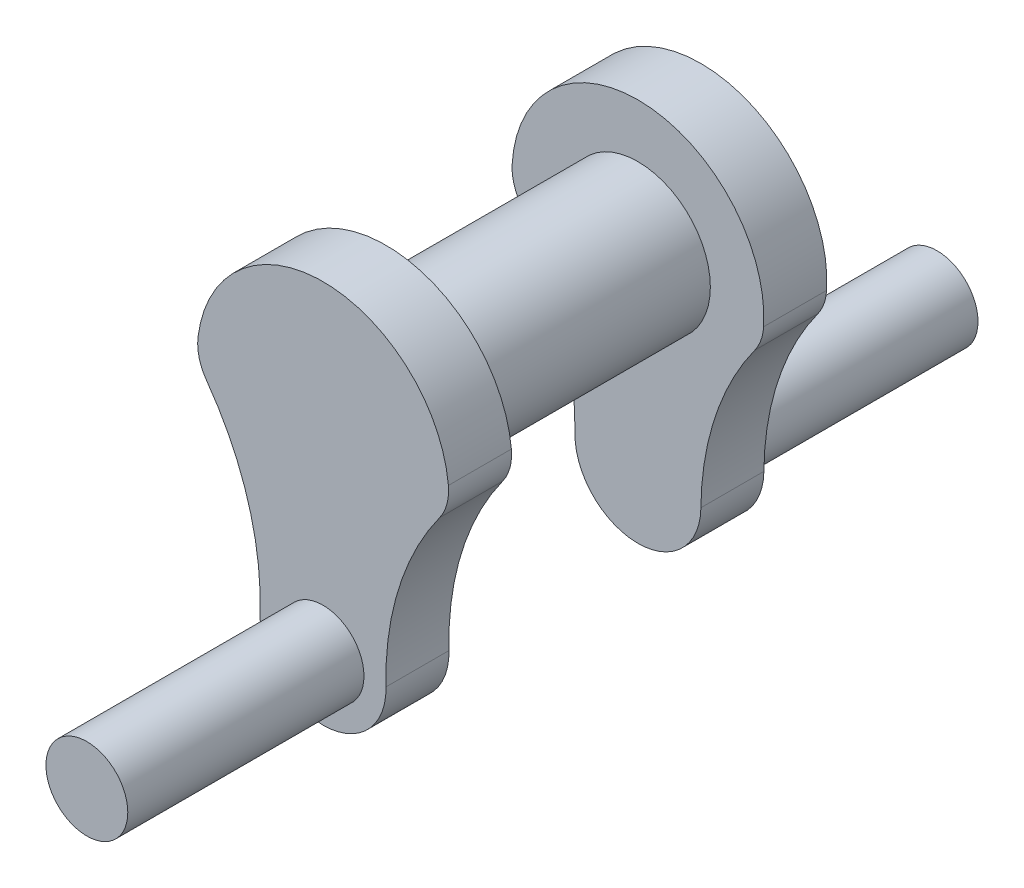
ISO-10303-21;
HEADER;
FILE_DESCRIPTION(('STEP AP214'),'2;1');
FILE_NAME('part.step','',(''),(''),'','','');
FILE_SCHEMA(('AUTOMOTIVE_DESIGN { 1 0 10303 214 1 1 1 1 }'));
ENDSEC;
DATA;
#1=APPLICATION_CONTEXT('core data for automotive mechanical design processes');
#2=APPLICATION_PROTOCOL_DEFINITION('international standard','automotive_design',2000,#1);
#3=PRODUCT_CONTEXT('',#1,'mechanical');
#4=PRODUCT('Part','Part','',(#3));
#5=PRODUCT_RELATED_PRODUCT_CATEGORY('part','',(#4));
#6=PRODUCT_DEFINITION_FORMATION('','',#4);
#7=PRODUCT_DEFINITION_CONTEXT('part definition',#1,'design');
#8=PRODUCT_DEFINITION('design','',#6,#7);
#9=PRODUCT_DEFINITION_SHAPE('','',#8);
#10=(LENGTH_UNIT() NAMED_UNIT(*) SI_UNIT(.MILLI.,.METRE.));
#11=(NAMED_UNIT(*) PLANE_ANGLE_UNIT() SI_UNIT($,.RADIAN.));
#12=(NAMED_UNIT(*) SI_UNIT($,.STERADIAN.) SOLID_ANGLE_UNIT());
#13=UNCERTAINTY_MEASURE_WITH_UNIT(LENGTH_MEASURE(1.E-05),#10,'distance_accuracy_value','');
#14=(GEOMETRIC_REPRESENTATION_CONTEXT(3) GLOBAL_UNCERTAINTY_ASSIGNED_CONTEXT((#13)) GLOBAL_UNIT_ASSIGNED_CONTEXT((#10,
#11,#12)) REPRESENTATION_CONTEXT('',''));
#15=CARTESIAN_POINT('',(0.,0.,0.));
#16=DIRECTION('',(0.,0.,1.));
#17=DIRECTION('',(1.,0.,0.));
#18=AXIS2_PLACEMENT_3D('',#15,#16,#17);
#19=CARTESIAN_POINT('',(-109.940604211098,3.61435273577438,20.));
#20=DIRECTION('',(0.,0.,-1.));
#21=DIRECTION('',(-1.,0.,0.));
#22=AXIS2_PLACEMENT_3D('',#19,#20,#21);
#23=CYLINDRICAL_SURFACE('',#22,90.);
#24=CARTESIAN_POINT('',(-109.940604211098,3.61435273577438,0.));
#25=DIRECTION('',(0.,0.,-1.));
#26=DIRECTION('',(1.,0.,0.));
#27=AXIS2_PLACEMENT_3D('',#24,#25,#26);
#28=CIRCLE('',#27,90.);
#29=CARTESIAN_POINT('',(-36.971364547257,56.2972727657126,0.));
#30=VERTEX_POINT('',#29);
#31=CARTESIAN_POINT('',(-19.9892007656543,0.657155042868067,0.));
#32=VERTEX_POINT('',#31);
#33=EDGE_CURVE('E126',#30,#32,#28,.T.);
#34=ORIENTED_EDGE('',*,*,#33,.T.);
#35=DIRECTION('',(0.,0.,-1.));
#36=VECTOR('',#35,1.);
#37=CARTESIAN_POINT('',(-19.9892007656543,0.657155042868067,20.));
#38=LINE('',#37,#36);
#39=CARTESIAN_POINT('',(-19.9892007656543,0.657155042868067,20.));
#40=VERTEX_POINT('',#39);
#41=EDGE_CURVE('E148',#40,#32,#38,.T.);
#42=ORIENTED_EDGE('',*,*,#41,.F.);
#43=CARTESIAN_POINT('',(-109.940604211098,3.61435273577438,20.));
#44=DIRECTION('',(0.,0.,-1.));
#45=DIRECTION('',(1.,0.,0.));
#46=AXIS2_PLACEMENT_3D('',#43,#44,#45);
#47=CIRCLE('',#46,90.);
#48=CARTESIAN_POINT('',(-36.971364547257,56.2972727657126,20.));
#49=VERTEX_POINT('',#48);
#50=EDGE_CURVE('E138',#49,#40,#47,.T.);
#51=ORIENTED_EDGE('',*,*,#50,.F.);
#52=DIRECTION('',(0.,0.,-1.));
#53=VECTOR('',#52,1.);
#54=CARTESIAN_POINT('',(-36.971364547257,56.2972727657126,20.));
#55=LINE('',#54,#53);
#56=EDGE_CURVE('E123',#49,#30,#55,.T.);
#57=ORIENTED_EDGE('',*,*,#56,.T.);
#58=EDGE_LOOP('',(#34,#42,#51,#57));
#59=FACE_BOUND('',#58,.T.);
#60=ADVANCED_FACE('F39',(#59),#23,.F.);
#61=CARTESIAN_POINT('',(0.,0.,20.));
#62=DIRECTION('',(0.,0.,-1.));
#63=DIRECTION('',(-1.,0.,0.));
#64=AXIS2_PLACEMENT_3D('',#61,#62,#63);
#65=CYLINDRICAL_SURFACE('',#64,20.);
#66=CARTESIAN_POINT('',(0.,0.,0.));
#67=DIRECTION('',(0.,0.,1.));
#68=DIRECTION('',(1.,0.,0.));
#69=AXIS2_PLACEMENT_3D('',#66,#67,#68);
#70=CIRCLE('',#69,20.);
#71=CARTESIAN_POINT('',(19.9931972894007,0.521595769827625,0.));
#72=VERTEX_POINT('',#71);
#73=EDGE_CURVE('E131',#32,#72,#70,.T.);
#74=ORIENTED_EDGE('',*,*,#73,.T.);
#75=DIRECTION('',(0.,0.,-1.));
#76=VECTOR('',#75,1.);
#77=CARTESIAN_POINT('',(19.9931972894007,0.521595769827625,20.));
#78=LINE('',#77,#76);
#79=CARTESIAN_POINT('',(19.9931972894007,0.521595769827625,20.));
#80=VERTEX_POINT('',#79);
#81=EDGE_CURVE('E141',#80,#72,#78,.T.);
#82=ORIENTED_EDGE('',*,*,#81,.F.);
#83=CARTESIAN_POINT('',(0.,0.,20.));
#84=DIRECTION('',(0.,0.,1.));
#85=DIRECTION('',(1.,0.,0.));
#86=AXIS2_PLACEMENT_3D('',#83,#84,#85);
#87=CIRCLE('',#86,20.);
#88=EDGE_CURVE('E94',#40,#80,#87,.T.);
#89=ORIENTED_EDGE('',*,*,#88,.F.);
#90=ORIENTED_EDGE('',*,*,#41,.T.);
#91=EDGE_LOOP('',(#74,#82,#89,#90));
#92=FACE_BOUND('',#91,.T.);
#93=ADVANCED_FACE('F172',(#92),#65,.T.);
#94=CARTESIAN_POINT('',(109.962585091704,2.86877673405191,20.));
#95=DIRECTION('',(0.,0.,-1.));
#96=DIRECTION('',(-1.,0.,0.));
#97=AXIS2_PLACEMENT_3D('',#94,#95,#96);
#98=CYLINDRICAL_SURFACE('',#97,90.);
#99=CARTESIAN_POINT('',(109.962585091704,2.86877673405191,0.));
#100=DIRECTION('',(0.,0.,-1.));
#101=DIRECTION('',(-1.,0.,0.));
#102=AXIS2_PLACEMENT_3D('',#99,#100,#101);
#103=CIRCLE('',#102,90.);
#104=CARTESIAN_POINT('',(37.038164849552,55.6137189782716,0.));
#105=VERTEX_POINT('',#104);
#106=EDGE_CURVE('E133',#72,#105,#103,.T.);
#107=ORIENTED_EDGE('',*,*,#106,.T.);
#108=DIRECTION('',(0.,0.,-1.));
#109=VECTOR('',#108,1.);
#110=CARTESIAN_POINT('',(37.038164849552,55.6137189782716,20.));
#111=LINE('',#110,#109);
#112=CARTESIAN_POINT('',(37.038164849552,55.6137189782716,20.));
#113=VERTEX_POINT('',#112);
#114=EDGE_CURVE('E118',#113,#105,#111,.T.);
#115=ORIENTED_EDGE('',*,*,#114,.F.);
#116=CARTESIAN_POINT('',(109.962585091704,2.86877673405191,20.));
#117=DIRECTION('',(0.,0.,-1.));
#118=DIRECTION('',(-1.,0.,0.));
#119=AXIS2_PLACEMENT_3D('',#116,#117,#118);
#120=CIRCLE('',#119,90.);
#121=EDGE_CURVE('E109',#80,#113,#120,.T.);
#122=ORIENTED_EDGE('',*,*,#121,.F.);
#123=ORIENTED_EDGE('',*,*,#81,.T.);
#124=EDGE_LOOP('',(#107,#115,#122,#123));
#125=FACE_BOUND('',#124,.T.);
#126=ADVANCED_FACE('F176',(#125),#98,.F.);
#127=CARTESIAN_POINT('',(24.8840948091934,64.4045426856415,20.));
#128=DIRECTION('',(0.,0.,-1.));
#129=DIRECTION('',(-1.,0.,0.));
#130=AXIS2_PLACEMENT_3D('',#127,#128,#129);
#131=CYLINDRICAL_SURFACE('',#130,15.);
#132=CARTESIAN_POINT('',(24.8840948091934,64.4045426856415,0.));
#133=DIRECTION('',(0.,0.,1.));
#134=DIRECTION('',(1.,0.,0.));
#135=AXIS2_PLACEMENT_3D('',#132,#133,#134);
#136=CIRCLE('',#135,15.);
#137=CARTESIAN_POINT('',(39.8145516947095,65.8472682970264,0.));
#138=VERTEX_POINT('',#137);
#139=EDGE_CURVE('E117',#105,#138,#136,.T.);
#140=ORIENTED_EDGE('',*,*,#139,.T.);
#141=DIRECTION('',(0.,0.,-1.));
#142=VECTOR('',#141,1.);
#143=CARTESIAN_POINT('',(39.8145516947095,65.8472682970264,20.));
#144=LINE('',#143,#142);
#145=CARTESIAN_POINT('',(39.8145516947095,65.8472682970264,20.));
#146=VERTEX_POINT('',#145);
#147=EDGE_CURVE('E113',#146,#138,#144,.T.);
#148=ORIENTED_EDGE('',*,*,#147,.F.);
#149=CARTESIAN_POINT('',(24.8840948091934,64.4045426856415,20.));
#150=DIRECTION('',(0.,0.,1.));
#151=DIRECTION('',(1.,0.,0.));
#152=AXIS2_PLACEMENT_3D('',#149,#150,#151);
#153=CIRCLE('',#152,15.);
#154=EDGE_CURVE('E102',#113,#146,#153,.T.);
#155=ORIENTED_EDGE('',*,*,#154,.F.);
#156=ORIENTED_EDGE('',*,*,#114,.T.);
#157=EDGE_LOOP('',(#140,#148,#155,#156));
#158=FACE_BOUND('',#157,.T.);
#159=ADVANCED_FACE('F116',(#158),#131,.T.);
#160=CARTESIAN_POINT('',(0.,62.,20.));
#161=DIRECTION('',(0.,0.,-1.));
#162=DIRECTION('',(-1.,0.,0.));
#163=AXIS2_PLACEMENT_3D('',#160,#161,#162);
#164=CYLINDRICAL_SURFACE('',#163,40.);
#165=CARTESIAN_POINT('',(0.,62.,0.));
#166=DIRECTION('',(0.,0.,1.));
#167=DIRECTION('',(1.,0.,0.));
#168=AXIS2_PLACEMENT_3D('',#165,#166,#167);
#169=CIRCLE('',#168,40.);
#170=CARTESIAN_POINT('',(-39.6957193652535,66.9244150997903,0.));
#171=VERTEX_POINT('',#170);
#172=EDGE_CURVE('E78',#138,#171,#169,.T.);
#173=ORIENTED_EDGE('',*,*,#172,.T.);
#174=DIRECTION('',(0.,0.,-1.));
#175=VECTOR('',#174,1.);
#176=CARTESIAN_POINT('',(-39.6957193652535,66.9244150997903,20.));
#177=LINE('',#176,#175);
#178=CARTESIAN_POINT('',(-39.6957193652535,66.9244150997903,20.));
#179=VERTEX_POINT('',#178);
#180=EDGE_CURVE('E119',#179,#171,#177,.T.);
#181=ORIENTED_EDGE('',*,*,#180,.F.);
#182=CARTESIAN_POINT('',(0.,62.,20.));
#183=DIRECTION('',(0.,0.,1.));
#184=DIRECTION('',(1.,0.,0.));
#185=AXIS2_PLACEMENT_3D('',#182,#183,#184);
#186=CIRCLE('',#185,40.);
#187=EDGE_CURVE('E107',#146,#179,#186,.T.);
#188=ORIENTED_EDGE('',*,*,#187,.F.);
#189=ORIENTED_EDGE('',*,*,#147,.T.);
#190=EDGE_LOOP('',(#173,#181,#188,#189));
#191=FACE_BOUND('',#190,.T.);
#192=ADVANCED_FACE('F121',(#191),#164,.T.);
#193=CARTESIAN_POINT('',(-24.8098246032834,65.077759437369,20.));
#194=DIRECTION('',(0.,0.,-1.));
#195=DIRECTION('',(-1.,0.,0.));
#196=AXIS2_PLACEMENT_3D('',#193,#194,#195);
#197=CYLINDRICAL_SURFACE('',#196,15.);
#198=CARTESIAN_POINT('',(-24.8098246032834,65.077759437369,0.));
#199=DIRECTION('',(0.,0.,1.));
#200=DIRECTION('',(1.,0.,0.));
#201=AXIS2_PLACEMENT_3D('',#198,#199,#200);
#202=CIRCLE('',#201,15.);
#203=EDGE_CURVE('E82',#171,#30,#202,.T.);
#204=ORIENTED_EDGE('',*,*,#203,.T.);
#205=ORIENTED_EDGE('',*,*,#56,.F.);
#206=CARTESIAN_POINT('',(-24.8098246032834,65.077759437369,20.));
#207=DIRECTION('',(0.,0.,1.));
#208=DIRECTION('',(1.,0.,0.));
#209=AXIS2_PLACEMENT_3D('',#206,#207,#208);
#210=CIRCLE('',#209,15.);
#211=EDGE_CURVE('E54',#179,#49,#210,.T.);
#212=ORIENTED_EDGE('',*,*,#211,.F.);
#213=ORIENTED_EDGE('',*,*,#180,.T.);
#214=EDGE_LOOP('',(#204,#205,#212,#213));
#215=FACE_BOUND('',#214,.T.);
#216=ADVANCED_FACE('F165',(#215),#197,.T.);
#217=CARTESIAN_POINT('',(-67.375214407191,34.3460560865717,20.));
#218=DIRECTION('',(0.,0.,1.));
#219=DIRECTION('',(1.,0.,0.));
#220=AXIS2_PLACEMENT_3D('',#217,#218,#219);
#221=PLANE('',#220);
#222=CARTESIAN_POINT('',(0.,0.,20.));
#223=DIRECTION('',(0.,0.,1.));
#224=DIRECTION('',(1.,0.,0.));
#225=AXIS2_PLACEMENT_3D('',#222,#223,#224);
#226=CIRCLE('',#225,13.);
#227=CARTESIAN_POINT('',(13.,0.,20.));
#228=VERTEX_POINT('',#227);
#229=EDGE_CURVE('E404',#228,#228,#226,.T.);
#230=ORIENTED_EDGE('',*,*,#229,.F.);
#231=EDGE_LOOP('',(#230));
#232=FACE_BOUND('',#231,.T.);
#233=ORIENTED_EDGE('',*,*,#50,.T.);
#234=ORIENTED_EDGE('',*,*,#88,.T.);
#235=ORIENTED_EDGE('',*,*,#121,.T.);
#236=ORIENTED_EDGE('',*,*,#154,.T.);
#237=ORIENTED_EDGE('',*,*,#187,.T.);
#238=ORIENTED_EDGE('',*,*,#211,.T.);
#239=EDGE_LOOP('',(#233,#234,#235,#236,#237,#238));
#240=FACE_BOUND('',#239,.T.);
#241=ADVANCED_FACE('F106',(#232,#240),#221,.T.);
#242=CARTESIAN_POINT('',(-67.375214407191,34.3460560865717,0.));
#243=DIRECTION('',(0.,0.,1.));
#244=DIRECTION('',(1.,0.,0.));
#245=AXIS2_PLACEMENT_3D('',#242,#243,#244);
#246=PLANE('',#245);
#247=CARTESIAN_POINT('',(0.,62.,0.));
#248=DIRECTION('',(0.,0.,1.));
#249=DIRECTION('',(1.,0.,0.));
#250=AXIS2_PLACEMENT_3D('',#247,#248,#249);
#251=CIRCLE('',#250,23.);
#252=CARTESIAN_POINT('',(23.,62.,0.));
#253=VERTEX_POINT('',#252);
#254=EDGE_CURVE('E50',#253,#253,#251,.F.);
#255=ORIENTED_EDGE('',*,*,#254,.F.);
#256=EDGE_LOOP('',(#255));
#257=FACE_BOUND('',#256,.T.);
#258=ORIENTED_EDGE('',*,*,#33,.F.);
#259=ORIENTED_EDGE('',*,*,#203,.F.);
#260=ORIENTED_EDGE('',*,*,#172,.F.);
#261=ORIENTED_EDGE('',*,*,#139,.F.);
#262=ORIENTED_EDGE('',*,*,#106,.F.);
#263=ORIENTED_EDGE('',*,*,#73,.F.);
#264=EDGE_LOOP('',(#258,#259,#260,#261,#262,#263));
#265=FACE_BOUND('',#264,.T.);
#266=ADVANCED_FACE('F155',(#257,#265),#246,.F.);
#267=CARTESIAN_POINT('',(0.,0.,95.));
#268=DIRECTION('',(0.,0.,-1.));
#269=DIRECTION('',(-1.,0.,0.));
#270=AXIS2_PLACEMENT_3D('',#267,#268,#269);
#271=CYLINDRICAL_SURFACE('',#270,13.);
#272=CARTESIAN_POINT('',(0.,0.,95.));
#273=DIRECTION('',(0.,0.,1.));
#274=DIRECTION('',(1.,0.,0.));
#275=AXIS2_PLACEMENT_3D('',#272,#273,#274);
#276=CIRCLE('',#275,13.);
#277=CARTESIAN_POINT('',(13.,0.,95.));
#278=VERTEX_POINT('',#277);
#279=EDGE_CURVE('E135',#278,#278,#276,.T.);
#280=ORIENTED_EDGE('',*,*,#279,.F.);
#281=EDGE_LOOP('',(#280));
#282=FACE_BOUND('',#281,.T.);
#283=ORIENTED_EDGE('',*,*,#229,.T.);
#284=EDGE_LOOP('',(#283));
#285=FACE_BOUND('',#284,.T.);
#286=ADVANCED_FACE('F154',(#282,#285),#271,.T.);
#287=CARTESIAN_POINT('',(0.,0.,95.));
#288=DIRECTION('',(0.,0.,1.));
#289=DIRECTION('',(1.,0.,0.));
#290=AXIS2_PLACEMENT_3D('',#287,#288,#289);
#291=PLANE('',#290);
#292=ORIENTED_EDGE('',*,*,#279,.T.);
#293=EDGE_LOOP('',(#292));
#294=FACE_BOUND('',#293,.T.);
#295=ADVANCED_FACE('F225',(#294),#291,.T.);
#296=CARTESIAN_POINT('',(0.,62.,-80.));
#297=DIRECTION('',(0.,0.,1.));
#298=DIRECTION('',(1.,0.,0.));
#299=AXIS2_PLACEMENT_3D('',#296,#297,#298);
#300=CYLINDRICAL_SURFACE('',#299,23.);
#301=CARTESIAN_POINT('',(0.,62.,-80.));
#302=DIRECTION('',(0.,0.,-1.));
#303=DIRECTION('',(-1.,0.,0.));
#304=AXIS2_PLACEMENT_3D('',#301,#302,#303);
#305=CIRCLE('',#304,23.);
#306=CARTESIAN_POINT('',(-23.,62.,-80.));
#307=VERTEX_POINT('',#306);
#308=EDGE_CURVE('E390',#307,#307,#305,.T.);
#309=ORIENTED_EDGE('',*,*,#308,.F.);
#310=EDGE_LOOP('',(#309));
#311=FACE_BOUND('',#310,.T.);
#312=ORIENTED_EDGE('',*,*,#254,.T.);
#313=EDGE_LOOP('',(#312));
#314=FACE_BOUND('',#313,.T.);
#315=ADVANCED_FACE('F147',(#311,#314),#300,.T.);
#316=CARTESIAN_POINT('',(-109.986288648504,1.73675252353752,-100.));
#317=DIRECTION('',(0.,0.,1.));
#318=DIRECTION('',(1.,0.,0.));
#319=AXIS2_PLACEMENT_3D('',#316,#317,#318);
#320=CYLINDRICAL_SURFACE('',#319,90.);
#321=CARTESIAN_POINT('',(-109.986288648504,1.73675252353752,-80.));
#322=DIRECTION('',(0.,0.,-1.));
#323=DIRECTION('',(1.,0.,0.));
#324=AXIS2_PLACEMENT_3D('',#321,#322,#323);
#325=CIRCLE('',#324,90.);
#326=CARTESIAN_POINT('',(-37.1096547179209,54.5477005073394,-80.));
#327=VERTEX_POINT('',#326);
#328=CARTESIAN_POINT('',(-19.9975070270007,0.315773186097732,-80.));
#329=VERTEX_POINT('',#328);
#330=EDGE_CURVE('E342',#327,#329,#325,.T.);
#331=ORIENTED_EDGE('',*,*,#330,.F.);
#332=DIRECTION('',(0.,0.,1.));
#333=VECTOR('',#332,1.);
#334=CARTESIAN_POINT('',(-37.1096547179209,54.5477005073394,-100.));
#335=LINE('',#334,#333);
#336=CARTESIAN_POINT('',(-37.1096547179209,54.5477005073394,-100.));
#337=VERTEX_POINT('',#336);
#338=EDGE_CURVE('E383',#337,#327,#335,.T.);
#339=ORIENTED_EDGE('',*,*,#338,.F.);
#340=CARTESIAN_POINT('',(-109.986288648504,1.73675252353752,-100.));
#341=DIRECTION('',(0.,0.,-1.));
#342=DIRECTION('',(1.,0.,0.));
#343=AXIS2_PLACEMENT_3D('',#340,#341,#342);
#344=CIRCLE('',#343,90.);
#345=CARTESIAN_POINT('',(-19.9975070270007,0.315773186097732,-100.));
#346=VERTEX_POINT('',#345);
#347=EDGE_CURVE('E351',#337,#346,#344,.T.);
#348=ORIENTED_EDGE('',*,*,#347,.T.);
#349=DIRECTION('',(0.,0.,1.));
#350=VECTOR('',#349,1.);
#351=CARTESIAN_POINT('',(-19.9975070270007,0.315773186097732,-100.));
#352=LINE('',#351,#350);
#353=EDGE_CURVE('E369',#346,#329,#352,.T.);
#354=ORIENTED_EDGE('',*,*,#353,.T.);
#355=EDGE_LOOP('',(#331,#339,#348,#354));
#356=FACE_BOUND('',#355,.T.);
#357=ADVANCED_FACE('F239',(#356),#320,.F.);
#358=CARTESIAN_POINT('',(-24.9635490628238,63.3495251713063,-100.));
#359=DIRECTION('',(0.,0.,1.));
#360=DIRECTION('',(1.,0.,0.));
#361=AXIS2_PLACEMENT_3D('',#358,#359,#360);
#362=CYLINDRICAL_SURFACE('',#361,15.);
#363=CARTESIAN_POINT('',(-24.9635490628238,63.3495251713063,-80.));
#364=DIRECTION('',(0.,0.,1.));
#365=DIRECTION('',(1.,0.,0.));
#366=AXIS2_PLACEMENT_3D('',#363,#364,#365);
#367=CIRCLE('',#366,15.);
#368=CARTESIAN_POINT('',(-39.9416785005181,64.1592402740902,-80.));
#369=VERTEX_POINT('',#368);
#370=EDGE_CURVE('E354',#369,#327,#367,.T.);
#371=ORIENTED_EDGE('',*,*,#370,.F.);
#372=DIRECTION('',(0.,0.,1.));
#373=VECTOR('',#372,1.);
#374=CARTESIAN_POINT('',(-39.9416785005181,64.1592402740902,-100.));
#375=LINE('',#374,#373);
#376=CARTESIAN_POINT('',(-39.9416785005181,64.1592402740902,-100.));
#377=VERTEX_POINT('',#376);
#378=EDGE_CURVE('E389',#377,#369,#375,.T.);
#379=ORIENTED_EDGE('',*,*,#378,.F.);
#380=CARTESIAN_POINT('',(-24.9635490628238,63.3495251713063,-100.));
#381=DIRECTION('',(0.,0.,1.));
#382=DIRECTION('',(1.,0.,0.));
#383=AXIS2_PLACEMENT_3D('',#380,#381,#382);
#384=CIRCLE('',#383,15.);
#385=EDGE_CURVE('E370',#377,#337,#384,.T.);
#386=ORIENTED_EDGE('',*,*,#385,.T.);
#387=ORIENTED_EDGE('',*,*,#338,.T.);
#388=EDGE_LOOP('',(#371,#379,#386,#387));
#389=FACE_BOUND('',#388,.T.);
#390=ADVANCED_FACE('F248',(#389),#362,.T.);
#391=CARTESIAN_POINT('',(0.,62.,-100.));
#392=DIRECTION('',(0.,0.,1.));
#393=DIRECTION('',(1.,0.,0.));
#394=AXIS2_PLACEMENT_3D('',#391,#392,#393);
#395=CYLINDRICAL_SURFACE('',#394,40.);
#396=CARTESIAN_POINT('',(0.,62.,-80.));
#397=DIRECTION('',(0.,0.,1.));
#398=DIRECTION('',(1.,0.,0.));
#399=AXIS2_PLACEMENT_3D('',#396,#397,#398);
#400=CIRCLE('',#399,40.);
#401=CARTESIAN_POINT('',(39.9242342726185,59.5392038391858,-80.));
#402=VERTEX_POINT('',#401);
#403=EDGE_CURVE('E377',#402,#369,#400,.T.);
#404=ORIENTED_EDGE('',*,*,#403,.F.);
#405=DIRECTION('',(0.,0.,1.));
#406=VECTOR('',#405,1.);
#407=CARTESIAN_POINT('',(39.9242342726185,59.5392038391858,-100.));
#408=LINE('',#407,#406);
#409=CARTESIAN_POINT('',(39.9242342726185,59.5392038391858,-100.));
#410=VERTEX_POINT('',#409);
#411=EDGE_CURVE('E391',#410,#402,#408,.T.);
#412=ORIENTED_EDGE('',*,*,#411,.F.);
#413=CARTESIAN_POINT('',(0.,62.,-100.));
#414=DIRECTION('',(0.,0.,1.));
#415=DIRECTION('',(1.,0.,0.));
#416=AXIS2_PLACEMENT_3D('',#413,#414,#415);
#417=CIRCLE('',#416,40.);
#418=EDGE_CURVE('E365',#410,#377,#417,.T.);
#419=ORIENTED_EDGE('',*,*,#418,.T.);
#420=ORIENTED_EDGE('',*,*,#378,.T.);
#421=EDGE_LOOP('',(#404,#412,#419,#420));
#422=FACE_BOUND('',#421,.T.);
#423=ADVANCED_FACE('F259',(#422),#395,.T.);
#424=CARTESIAN_POINT('',(24.9526464203865,60.4620023994912,-100.));
#425=DIRECTION('',(0.,0.,1.));
#426=DIRECTION('',(1.,0.,0.));
#427=AXIS2_PLACEMENT_3D('',#424,#425,#426);
#428=CYLINDRICAL_SURFACE('',#427,15.);
#429=CARTESIAN_POINT('',(24.9526464203865,60.4620023994912,-80.));
#430=DIRECTION('',(0.,0.,1.));
#431=DIRECTION('',(1.,0.,0.));
#432=AXIS2_PLACEMENT_3D('',#429,#430,#431);
#433=CIRCLE('',#432,15.);
#434=CARTESIAN_POINT('',(37.10144689777,51.663897662633,-80.));
#435=VERTEX_POINT('',#434);
#436=EDGE_CURVE('E376',#435,#402,#433,.T.);
#437=ORIENTED_EDGE('',*,*,#436,.F.);
#438=DIRECTION('',(0.,0.,1.));
#439=VECTOR('',#438,1.);
#440=CARTESIAN_POINT('',(37.10144689777,51.663897662633,-100.));
#441=LINE('',#440,#439);
#442=CARTESIAN_POINT('',(37.10144689777,51.663897662633,-100.));
#443=VERTEX_POINT('',#442);
#444=EDGE_CURVE('E393',#443,#435,#441,.T.);
#445=ORIENTED_EDGE('',*,*,#444,.F.);
#446=CARTESIAN_POINT('',(24.9526464203865,60.4620023994912,-100.));
#447=DIRECTION('',(0.,0.,1.));
#448=DIRECTION('',(1.,0.,0.));
#449=AXIS2_PLACEMENT_3D('',#446,#447,#448);
#450=CIRCLE('',#449,15.);
#451=EDGE_CURVE('E363',#443,#410,#450,.T.);
#452=ORIENTED_EDGE('',*,*,#451,.T.);
#453=ORIENTED_EDGE('',*,*,#411,.T.);
#454=EDGE_LOOP('',(#437,#445,#452,#453));
#455=FACE_BOUND('',#454,.T.);
#456=ADVANCED_FACE('F267',(#455),#428,.T.);
#457=CARTESIAN_POINT('',(109.994249762071,-1.12473075851625,-100.));
#458=DIRECTION('',(0.,0.,1.));
#459=DIRECTION('',(1.,0.,0.));
#460=AXIS2_PLACEMENT_3D('',#457,#458,#459);
#461=CYLINDRICAL_SURFACE('',#460,90.);
#462=CARTESIAN_POINT('',(109.994249762071,-1.12473075851625,-80.));
#463=DIRECTION('',(0.,0.,-1.));
#464=DIRECTION('',(1.,0.,0.));
#465=AXIS2_PLACEMENT_3D('',#462,#463,#464);
#466=CIRCLE('',#465,90.);
#467=CARTESIAN_POINT('',(19.9989545021947,-0.204496501548406,-80.));
#468=VERTEX_POINT('',#467);
#469=EDGE_CURVE('E373',#468,#435,#466,.T.);
#470=ORIENTED_EDGE('',*,*,#469,.F.);
#471=DIRECTION('',(0.,0.,1.));
#472=VECTOR('',#471,1.);
#473=CARTESIAN_POINT('',(19.9989545021947,-0.204496501548406,-100.));
#474=LINE('',#473,#472);
#475=CARTESIAN_POINT('',(19.9989545021947,-0.204496501548406,-100.));
#476=VERTEX_POINT('',#475);
#477=EDGE_CURVE('E396',#476,#468,#474,.T.);
#478=ORIENTED_EDGE('',*,*,#477,.F.);
#479=CARTESIAN_POINT('',(109.994249762071,-1.12473075851625,-100.));
#480=DIRECTION('',(0.,0.,-1.));
#481=DIRECTION('',(1.,0.,0.));
#482=AXIS2_PLACEMENT_3D('',#479,#480,#481);
#483=CIRCLE('',#482,90.);
#484=EDGE_CURVE('E360',#476,#443,#483,.T.);
#485=ORIENTED_EDGE('',*,*,#484,.T.);
#486=ORIENTED_EDGE('',*,*,#444,.T.);
#487=EDGE_LOOP('',(#470,#478,#485,#486));
#488=FACE_BOUND('',#487,.T.);
#489=ADVANCED_FACE('F276',(#488),#461,.F.);
#490=CARTESIAN_POINT('',(0.,0.,-100.));
#491=DIRECTION('',(0.,0.,1.));
#492=DIRECTION('',(1.,0.,0.));
#493=AXIS2_PLACEMENT_3D('',#490,#491,#492);
#494=CYLINDRICAL_SURFACE('',#493,20.);
#495=CARTESIAN_POINT('',(0.,0.,-80.));
#496=DIRECTION('',(0.,0.,1.));
#497=DIRECTION('',(1.,0.,0.));
#498=AXIS2_PLACEMENT_3D('',#495,#496,#497);
#499=CIRCLE('',#498,20.);
#500=EDGE_CURVE('E346',#329,#468,#499,.T.);
#501=ORIENTED_EDGE('',*,*,#500,.F.);
#502=ORIENTED_EDGE('',*,*,#353,.F.);
#503=CARTESIAN_POINT('',(0.,0.,-100.));
#504=DIRECTION('',(0.,0.,1.));
#505=DIRECTION('',(1.,0.,0.));
#506=AXIS2_PLACEMENT_3D('',#503,#504,#505);
#507=CIRCLE('',#506,20.);
#508=EDGE_CURVE('E353',#346,#476,#507,.T.);
#509=ORIENTED_EDGE('',*,*,#508,.T.);
#510=ORIENTED_EDGE('',*,*,#477,.T.);
#511=EDGE_LOOP('',(#501,#502,#509,#510));
#512=FACE_BOUND('',#511,.T.);
#513=ADVANCED_FACE('F288',(#512),#494,.T.);
#514=CARTESIAN_POINT('',(-67.4749188556638,32.5431388474219,-100.));
#515=DIRECTION('',(0.,0.,1.));
#516=DIRECTION('',(1.,0.,0.));
#517=AXIS2_PLACEMENT_3D('',#514,#515,#516);
#518=PLANE('',#517);
#519=CARTESIAN_POINT('',(0.,0.,-100.));
#520=DIRECTION('',(0.,0.,1.));
#521=DIRECTION('',(1.,0.,0.));
#522=AXIS2_PLACEMENT_3D('',#519,#520,#521);
#523=CIRCLE('',#522,13.);
#524=CARTESIAN_POINT('',(13.,0.,-100.));
#525=VERTEX_POINT('',#524);
#526=EDGE_CURVE('E11',#525,#525,#523,.F.);
#527=ORIENTED_EDGE('',*,*,#526,.F.);
#528=EDGE_LOOP('',(#527));
#529=FACE_BOUND('',#528,.T.);
#530=ORIENTED_EDGE('',*,*,#347,.F.);
#531=ORIENTED_EDGE('',*,*,#385,.F.);
#532=ORIENTED_EDGE('',*,*,#418,.F.);
#533=ORIENTED_EDGE('',*,*,#451,.F.);
#534=ORIENTED_EDGE('',*,*,#484,.F.);
#535=ORIENTED_EDGE('',*,*,#508,.F.);
#536=EDGE_LOOP('',(#530,#531,#532,#533,#534,#535));
#537=FACE_BOUND('',#536,.T.);
#538=ADVANCED_FACE('F298',(#529,#537),#518,.F.);
#539=CARTESIAN_POINT('',(-67.4749188556638,32.5431388474219,-80.));
#540=DIRECTION('',(0.,0.,1.));
#541=DIRECTION('',(1.,0.,0.));
#542=AXIS2_PLACEMENT_3D('',#539,#540,#541);
#543=PLANE('',#542);
#544=ORIENTED_EDGE('',*,*,#308,.T.);
#545=EDGE_LOOP('',(#544));
#546=FACE_BOUND('',#545,.T.);
#547=ORIENTED_EDGE('',*,*,#330,.T.);
#548=ORIENTED_EDGE('',*,*,#500,.T.);
#549=ORIENTED_EDGE('',*,*,#469,.T.);
#550=ORIENTED_EDGE('',*,*,#436,.T.);
#551=ORIENTED_EDGE('',*,*,#403,.T.);
#552=ORIENTED_EDGE('',*,*,#370,.T.);
#553=EDGE_LOOP('',(#547,#548,#549,#550,#551,#552));
#554=FACE_BOUND('',#553,.T.);
#555=ADVANCED_FACE('F309',(#546,#554),#543,.T.);
#556=CARTESIAN_POINT('',(0.,0.,-175.));
#557=DIRECTION('',(0.,0.,1.));
#558=DIRECTION('',(1.,0.,0.));
#559=AXIS2_PLACEMENT_3D('',#556,#557,#558);
#560=CYLINDRICAL_SURFACE('',#559,13.);
#561=CARTESIAN_POINT('',(0.,0.,-175.));
#562=DIRECTION('',(0.,0.,-1.));
#563=DIRECTION('',(-1.,0.,0.));
#564=AXIS2_PLACEMENT_3D('',#561,#562,#563);
#565=CIRCLE('',#564,13.);
#566=CARTESIAN_POINT('',(-13.,0.,-175.));
#567=VERTEX_POINT('',#566);
#568=EDGE_CURVE('E343',#567,#567,#565,.T.);
#569=ORIENTED_EDGE('',*,*,#568,.F.);
#570=EDGE_LOOP('',(#569));
#571=FACE_BOUND('',#570,.T.);
#572=ORIENTED_EDGE('',*,*,#526,.T.);
#573=EDGE_LOOP('',(#572));
#574=FACE_BOUND('',#573,.T.);
#575=ADVANCED_FACE('F319',(#571,#574),#560,.T.);
#576=CARTESIAN_POINT('',(0.,0.,-175.));
#577=DIRECTION('',(0.,0.,-1.));
#578=DIRECTION('',(-1.,0.,0.));
#579=AXIS2_PLACEMENT_3D('',#576,#577,#578);
#580=PLANE('',#579);
#581=ORIENTED_EDGE('',*,*,#568,.T.);
#582=EDGE_LOOP('',(#581));
#583=FACE_BOUND('',#582,.T.);
#584=ADVANCED_FACE('F328',(#583),#580,.T.);
#585=CLOSED_SHELL('',(#60,#93,#126,#159,#192,#216,#241,#266,#286,#295,#315,#357,#390,#423,#456,
#489,#513,#538,#555,#575,#584));
#586=MANIFOLD_SOLID_BREP('B2',#585);
#587=ADVANCED_BREP_SHAPE_REPRESENTATION('',(#18,#586),#14);
#588=SHAPE_DEFINITION_REPRESENTATION(#9,#587);
ENDSEC;
END-ISO-10303-21;
